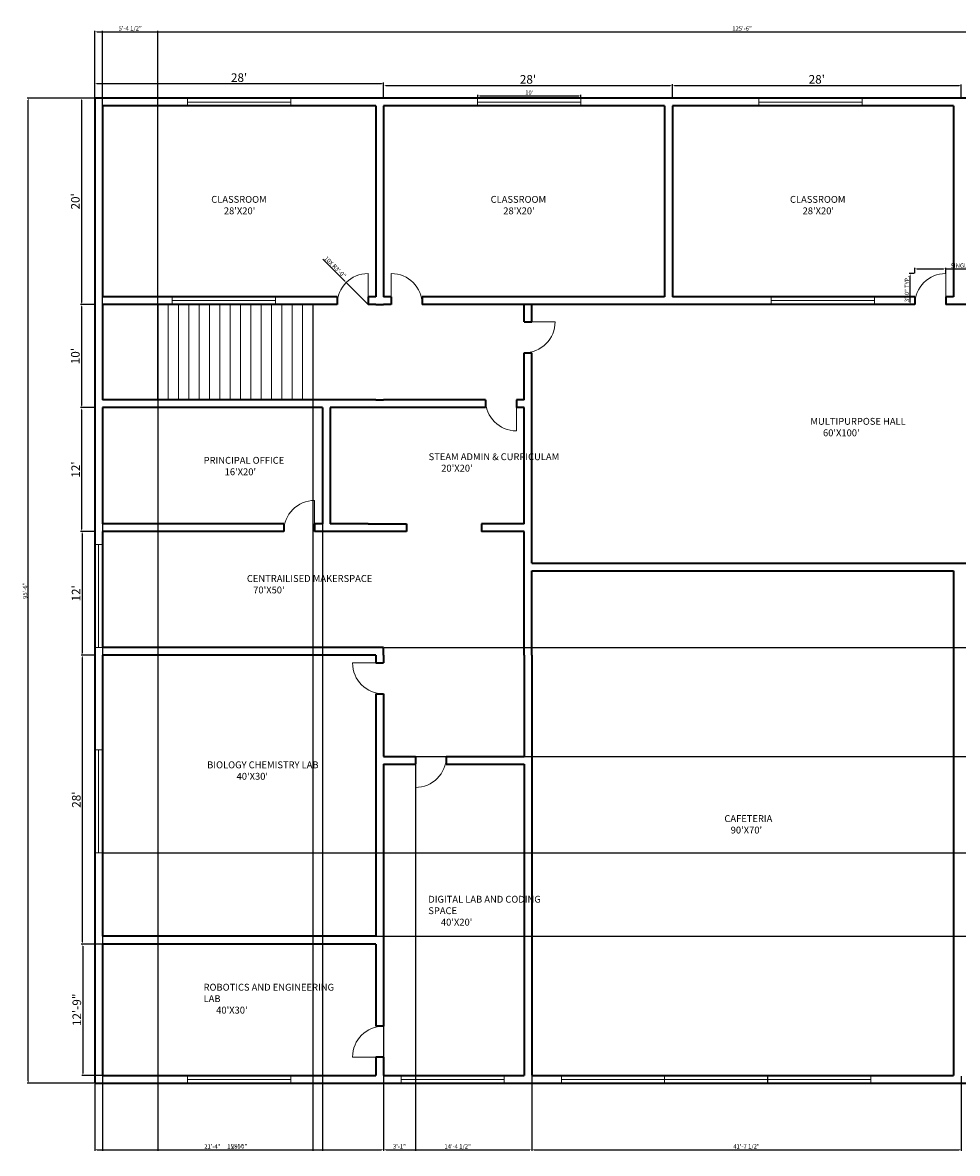
# Model space of a CAD drawing. Units: inches. Extents: x 2394 to 4066, y 1878 to 3193.
# Tile 1 of 3: x 2394 to 3482, y 1878 to 3193. Entities that reach past the tile are written whole.
import ezdxf

# ---------------------------------------------------------------- set-up
doc = ezdxf.new("R2010")
doc.units = ezdxf.units.IN
for name, color, linetype, lineweight in [('A-ANNO-DIMS', 2, 'Continuous', 13), ('A-AREA-IDEN', 7, 'Continuous', 18), ('A-DOOR', 3, 'Continuous', 18), ('A-FLOR-STRS', 8, 'Continuous', 18), ('A-GLAZ', 4, 'Continuous', 18), ('A-WALL', 7, 'Continuous', 35)]:
    doc.layers.add(name, color=color, linetype=linetype, lineweight=lineweight)
doc.styles.get("Standard").update_dxf_attribs({"font": 'arial.ttf'})
doc.dimstyles.new('ISO-25', dxfattribs={"dimtxt": 5, "dimasz": 2.5, "dimexe": 1.25, "dimexo": 0.625, "dimtad": 1, "dimlunit": 3, "dimtxsty": 'Standard', "dimcen": 2.5, "dimadec": 0, "dimazin": 0, "dimtfac": 1, "dimtmove": 0, "dimatfit": 3, "dimfxl": 1, "dimarcsym": 0})

# ---------------------------------------------------------------- blocks, each defined once
blk = doc.blocks.new('*D1')
at = {"layer": 'A-ANNO-DIMS', "color": 0, "lineweight": -2, "transparency": 16777216}
for p, q in [((2478.1, 3105.7), (2478.1, 3123.2)), ((2480.6, 3122), (2811.6, 3122)), ((2814.1, 3105.7), (2814.1, 3123.2))]:
    blk.add_line(p, q, dxfattribs=at)
at = {"layer": 'A-ANNO-DIMS', "color": 0, "transparency": 16777216}
for points in [[(2480.6, 3122.4), (2480.6, 3121.6), (2478.1, 3122)], [(2811.6, 3122.4), (2811.6, 3121.6), (2814.1, 3122)]]:
    blk.add_solid(points, dxfattribs=at)
at = {"layer": 'Defpoints', "color": 0, "transparency": 16777216}
for p in [(2814.1, 3122), (2478.1, 3105.1), (2814.1, 3105.1)]:
    blk.add_point(p, dxfattribs=at)
at = {"layer": 'A-ANNO-DIMS', "color": 0, "transparency": 16777216, "insert": (2646.1, 3127.7), "char_height": 10, "attachment_point": 5}
blk.add_mtext("28'", dxfattribs=at)
blk = doc.blocks.new('*D2')
at = {"layer": 'A-ANNO-DIMS', "color": 0, "lineweight": -2, "transparency": 16777216}
for p, q in [((2814.1, 3105.7), (2814.1, 3121.3)), ((2816.6, 3120), (3147.6, 3120)), ((3150.1, 3105.7), (3150.1, 3121.3))]:
    blk.add_line(p, q, dxfattribs=at)
at = {"layer": 'A-ANNO-DIMS', "color": 0, "transparency": 16777216}
for points in [[(2816.6, 3120.4), (2816.6, 3119.6), (2814.1, 3120)], [(3147.6, 3120.4), (3147.6, 3119.6), (3150.1, 3120)]]:
    blk.add_solid(points, dxfattribs=at)
at = {"layer": 'Defpoints', "color": 0, "transparency": 16777216}
for p in [(3150.1, 3120), (2814.1, 3105.1), (3150.1, 3105.1)]:
    blk.add_point(p, dxfattribs=at)
at = {"layer": 'A-ANNO-DIMS', "color": 0, "transparency": 16777216, "insert": (2982.1, 3125.7), "char_height": 10, "attachment_point": 5}
blk.add_mtext("28'", dxfattribs=at)
blk = doc.blocks.new('*D3')
at = {"layer": 'A-ANNO-DIMS', "color": 0, "lineweight": -2, "transparency": 16777216}
for p, q in [((3150.1, 3105.7), (3150.1, 3121.2)), ((3152.6, 3120), (3483.6, 3120)), ((3486.1, 3105.7), (3486.1, 3121.2))]:
    blk.add_line(p, q, dxfattribs=at)
at = {"layer": 'A-ANNO-DIMS', "color": 0, "transparency": 16777216}
for points in [[(3152.6, 3120.4), (3152.6, 3119.6), (3150.1, 3120)], [(3483.6, 3120.4), (3483.6, 3119.6), (3486.1, 3120)]]:
    blk.add_solid(points, dxfattribs=at)
at = {"layer": 'Defpoints', "color": 0, "transparency": 16777216}
for p in [(3486.1, 3120), (3150.1, 3105.1), (3486.1, 3105.1)]:
    blk.add_point(p, dxfattribs=at)
at = {"layer": 'A-ANNO-DIMS', "color": 0, "transparency": 16777216, "insert": (3318.1, 3125.7), "char_height": 10, "attachment_point": 5}
blk.add_mtext("28'", dxfattribs=at)
blk = doc.blocks.new('*D6')
at = {"layer": 'A-ANNO-DIMS', "color": 0, "lineweight": -2, "transparency": 16777216}
for p, q in [((2477.5, 3105.1), (2461.4, 3105.1)), ((2462.6, 3102.6), (2462.6, 2867.6)), ((2477.5, 2865.1), (2461.4, 2865.1))]:
    blk.add_line(p, q, dxfattribs=at)
at = {"layer": 'A-ANNO-DIMS', "color": 0, "transparency": 16777216}
for points in [[(2462.2, 3102.6), (2463, 3102.6), (2462.6, 3105.1)], [(2462.2, 2867.6), (2463, 2867.6), (2462.6, 2865.1)]]:
    blk.add_solid(points, dxfattribs=at)
at = {"layer": 'Defpoints', "color": 0, "transparency": 16777216}
for p in [(2478.1, 3105.1), (2462.6, 2865.1), (2478.1, 2865.1)]:
    blk.add_point(p, dxfattribs=at)
at = {"layer": 'A-ANNO-DIMS', "color": 0, "transparency": 16777216, "insert": (2456.9, 2985.1), "char_height": 10, "attachment_point": 5, "rotation": 90}
blk.add_mtext("20'", dxfattribs=at)
blk = doc.blocks.new('*D7')
at = {"layer": 'A-ANNO-DIMS', "color": 0, "lineweight": -2, "transparency": 16777216}
for p, q in [((2477.5, 2865.1), (2461.4, 2865.1)), ((2462.6, 2862.6), (2462.6, 2747.6)), ((2477.5, 2745.1), (2461.4, 2745.1))]:
    blk.add_line(p, q, dxfattribs=at)
at = {"layer": 'A-ANNO-DIMS', "color": 0, "transparency": 16777216}
for points in [[(2462.2, 2862.6), (2463, 2862.6), (2462.6, 2865.1)], [(2462.2, 2747.6), (2463, 2747.6), (2462.6, 2745.1)]]:
    blk.add_solid(points, dxfattribs=at)
at = {"layer": 'Defpoints', "color": 0, "transparency": 16777216}
for p in [(2478.1, 2865.1), (2462.6, 2745.1), (2478.1, 2745.1)]:
    blk.add_point(p, dxfattribs=at)
at = {"layer": 'A-ANNO-DIMS', "color": 0, "transparency": 16777216, "insert": (2456.9, 2805.1), "char_height": 10, "attachment_point": 5, "rotation": 90}
blk.add_mtext("10'", dxfattribs=at)
blk = doc.blocks.new('*D8')
at = {"layer": 'A-ANNO-DIMS', "color": 0, "lineweight": -2, "transparency": 16777216}
for p, q in [((2477.5, 2745.1), (2461.7, 2745.1)), ((2462.9, 2742.6), (2462.9, 2603.6)), ((2477.5, 2601.1), (2461.7, 2601.1))]:
    blk.add_line(p, q, dxfattribs=at)
at = {"layer": 'A-ANNO-DIMS', "color": 0, "transparency": 16777216}
for points in [[(2462.5, 2742.6), (2463.3, 2742.6), (2462.9, 2745.1)], [(2462.5, 2603.6), (2463.3, 2603.6), (2462.9, 2601.1)]]:
    blk.add_solid(points, dxfattribs=at)
at = {"layer": 'Defpoints', "color": 0, "transparency": 16777216}
for p in [(2478.1, 2745.1), (2462.9, 2601.1), (2478.1, 2601.1)]:
    blk.add_point(p, dxfattribs=at)
at = {"layer": 'A-ANNO-DIMS', "color": 0, "transparency": 16777216, "insert": (2457.3, 2673.1), "char_height": 10, "attachment_point": 5, "rotation": 90}
blk.add_mtext("12'", dxfattribs=at)
blk = doc.blocks.new('*D9')
at = {"layer": 'A-ANNO-DIMS', "color": 0, "lineweight": -2, "transparency": 16777216}
for p, q in [((2477.5, 2601.1), (2462.2, 2601.1)), ((2463.4, 2598.6), (2463.4, 2459.6)), ((2477.5, 2457.1), (2462.2, 2457.1))]:
    blk.add_line(p, q, dxfattribs=at)
at = {"layer": 'A-ANNO-DIMS', "color": 0, "transparency": 16777216}
for points in [[(2463, 2598.6), (2463.9, 2598.6), (2463.4, 2601.1)], [(2463, 2459.6), (2463.9, 2459.6), (2463.4, 2457.1)]]:
    blk.add_solid(points, dxfattribs=at)
at = {"layer": 'Defpoints', "color": 0, "transparency": 16777216}
for p in [(2478.1, 2601.1), (2463.4, 2457.1), (2478.1, 2457.1)]:
    blk.add_point(p, dxfattribs=at)
at = {"layer": 'A-ANNO-DIMS', "color": 0, "transparency": 16777216, "insert": (2457.8, 2529.1), "char_height": 10, "attachment_point": 5, "rotation": 90}
blk.add_mtext("12'", dxfattribs=at)
blk = doc.blocks.new('*D10')
at = {"layer": 'A-ANNO-DIMS', "color": 0, "lineweight": -2, "transparency": 16777216}
for p, q in [((2477.5, 2457.1), (2462.4, 2457.1)), ((2463.7, 2454.6), (2463.7, 2123.6)), ((2477.5, 2121.1), (2462.4, 2121.1))]:
    blk.add_line(p, q, dxfattribs=at)
at = {"layer": 'A-ANNO-DIMS', "color": 0, "transparency": 16777216}
for points in [[(2463.3, 2454.6), (2464.1, 2454.6), (2463.7, 2457.1)], [(2463.3, 2123.6), (2464.1, 2123.6), (2463.7, 2121.1)]]:
    blk.add_solid(points, dxfattribs=at)
at = {"layer": 'Defpoints', "color": 0, "transparency": 16777216}
for p in [(2478.1, 2457.1), (2463.7, 2121.1), (2478.1, 2121.1)]:
    blk.add_point(p, dxfattribs=at)
at = {"layer": 'A-ANNO-DIMS', "color": 0, "transparency": 16777216, "insert": (2458, 2289.1), "char_height": 10, "attachment_point": 5, "rotation": 90}
blk.add_mtext("28'", dxfattribs=at)
blk = doc.blocks.new('*D11')
at = {"layer": 'A-ANNO-DIMS', "color": 0, "lineweight": -2, "transparency": 16777216}
for p, q in [((2486.5, 2121.1), (2463, 2121.1)), ((2464.3, 2118.6), (2464.3, 1970.6)), ((2486.5, 1968.1), (2463, 1968.1))]:
    blk.add_line(p, q, dxfattribs=at)
at = {"layer": 'A-ANNO-DIMS', "color": 0, "transparency": 16777216}
for points in [[(2463.9, 2118.6), (2464.7, 2118.6), (2464.3, 2121.1)], [(2463.9, 1970.6), (2464.7, 1970.6), (2464.3, 1968.1)]]:
    blk.add_solid(points, dxfattribs=at)
at = {"layer": 'Defpoints', "color": 0, "transparency": 16777216}
for p in [(2487.1, 2121.1), (2464.3, 1968.1), (2487.1, 1968.1)]:
    blk.add_point(p, dxfattribs=at)
at = {"layer": 'A-ANNO-DIMS', "color": 0, "transparency": 16777216, "insert": (2458.6, 2044.6), "char_height": 10, "attachment_point": 5, "rotation": 90}
blk.add_mtext('12\'-9"', dxfattribs=at)
blk = doc.blocks.new('*D12')
at = {"layer": 'A-ANNO-DIMS', "color": 0, "lineweight": -2, "transparency": 16777216}
for p, q in [((2923.6, 3105.7), (2923.6, 3109)), ((2926.1, 3107.8), (3041.1, 3107.8)), ((3043.6, 3105.7), (3043.6, 3109))]:
    blk.add_line(p, q, dxfattribs=at)
at = {"layer": 'A-ANNO-DIMS', "color": 0, "transparency": 16777216}
for points in [[(2926.1, 3108.2), (2926.1, 3107.3), (2923.6, 3107.8)], [(3041.1, 3108.2), (3041.1, 3107.3), (3043.6, 3107.8)]]:
    blk.add_solid(points, dxfattribs=at)
at = {"layer": 'Defpoints', "color": 0, "transparency": 16777216}
for p in [(2923.6, 3105.1), (3043.6, 3107.8), (3043.6, 3105.1)]:
    blk.add_point(p, dxfattribs=at)
at = {"layer": 'A-ANNO-DIMS', "color": 0, "transparency": 16777216, "insert": (2983.6, 3110.9), "char_height": 5, "attachment_point": 5}
blk.add_mtext("10'", dxfattribs=at)
blk = doc.blocks.new('DOOR-SINGLE-36IN')
blk.add_line((36, 0), (36, 36))
blk.add_arc((36, 0), 36, 90, 180)
blk = doc.blocks.new('WINDOW-120IN')
for p, q in [((0, 0), (0, 9)), ((120, 4.5), (0, 4.5)), ((120, 0), (120, 9))]:
    blk.add_line(p, q)
blk = doc.blocks.new('*D15')
at = {"layer": 'A-ANNO-DIMS', "color": 0, "lineweight": -2, "transparency": 16777216}
for p, q in [((3432.1, 2901.7), (3432.1, 2907.7)), ((3468.1, 2901.7), (3468.1, 2907.7)), ((3434.6, 2906.5), (3465.6, 2906.5)), ((3468.1, 2906.5), (3552.8, 2906.5))]:
    blk.add_line(p, q, dxfattribs=at)
at = {"layer": 'A-ANNO-DIMS', "color": 0, "transparency": 16777216}
for points in [[(3434.6, 2906.9), (3434.6, 2906.1), (3432.1, 2906.5)], [(3465.6, 2906.9), (3465.6, 2906.1), (3468.1, 2906.5)]]:
    blk.add_solid(points, dxfattribs=at)
at = {"layer": 'Defpoints', "color": 0, "transparency": 16777216}
for p in [(3432.1, 2901.1), (3468.1, 2906.5), (3468.1, 2901.1)]:
    blk.add_point(p, dxfattribs=at)
at = {"layer": 'A-ANNO-DIMS', "color": 0, "transparency": 16777216, "insert": (3511.7, 2909.7), "char_height": 5, "attachment_point": 5}
blk.add_mtext('SINGLE DOOR 3\'-0" TYP.', dxfattribs=at)
blk = doc.blocks.new('*D16')
at = {"layer": 'A-ANNO-DIMS', "color": 0, "lineweight": -2, "transparency": 16777216}
for p, q in [((3431.5, 2901.1), (3425.4, 2901.1)), ((3426.7, 2867.6), (3426.7, 2898.6)), ((3431.5, 2865.1), (3425.4, 2865.1))]:
    blk.add_line(p, q, dxfattribs=at)
at = {"layer": 'A-ANNO-DIMS', "color": 0, "transparency": 16777216}
for points in [[(3426.3, 2898.6), (3427.1, 2898.6), (3426.7, 2901.1)], [(3426.3, 2867.6), (3427.1, 2867.6), (3426.7, 2865.1)]]:
    blk.add_solid(points, dxfattribs=at)
at = {"layer": 'Defpoints', "color": 0, "transparency": 16777216}
for p in [(3426.7, 2901.1), (3432.1, 2901.1), (3432.1, 2865.1)]:
    blk.add_point(p, dxfattribs=at)
at = {"layer": 'A-ANNO-DIMS', "color": 0, "transparency": 16777216, "insert": (3423.5, 2883.1), "char_height": 5, "attachment_point": 5, "rotation": 90}
blk.add_mtext('3\'-0" TYP.', dxfattribs=at)
blk = doc.blocks.new('*D19')
at = {"layer": 'A-ANNO-DIMS', "color": 0, "lineweight": -2, "transparency": 16777216}
for p, q in [((2478.1, 3105.7), (2478.1, 3183.6)), ((3984.1, 3105.7), (3984.1, 3183.6)), ((2480.6, 3182.3), (3981.6, 3182.3))]:
    blk.add_line(p, q, dxfattribs=at)
at = {"layer": 'A-ANNO-DIMS', "color": 0, "transparency": 16777216}
for points in [[(2480.6, 3182.8), (2480.6, 3181.9), (2478.1, 3182.3)], [(3981.6, 3182.8), (3981.6, 3181.9), (3984.1, 3182.3)]]:
    blk.add_solid(points, dxfattribs=at)
at = {"layer": 'Defpoints', "color": 0, "transparency": 16777216}
for p in [(3984.1, 3182.3), (2478.1, 3105.1), (3984.1, 3105.1)]:
    blk.add_point(p, dxfattribs=at)
at = {"layer": 'A-ANNO-DIMS', "color": 0, "transparency": 16777216, "insert": (3231.1, 3185.5), "char_height": 5, "attachment_point": 5}
blk.add_mtext('125\'-6"', dxfattribs=at)
blk = doc.blocks.new('*D20')
at = {"layer": 'A-ANNO-DIMS', "color": 0, "lineweight": -2, "transparency": 16777216}
for p, q in [((2477.5, 3105.1), (2399.6, 3105.1)), ((2400.8, 1961.6), (2400.8, 3102.6)), ((2477.5, 1959.1), (2399.6, 1959.1))]:
    blk.add_line(p, q, dxfattribs=at)
at = {"layer": 'A-ANNO-DIMS', "color": 0, "transparency": 16777216}
for points in [[(2400.4, 3102.6), (2401.3, 3102.6), (2400.8, 3105.1)], [(2400.4, 1961.6), (2401.3, 1961.6), (2400.8, 1959.1)]]:
    blk.add_solid(points, dxfattribs=at)
at = {"layer": 'Defpoints', "color": 0, "transparency": 16777216}
for p in [(2400.8, 3105.1), (2478.1, 3105.1), (2478.1, 1959.1)]:
    blk.add_point(p, dxfattribs=at)
at = {"layer": 'A-ANNO-DIMS', "color": 0, "transparency": 16777216, "insert": (2397.7, 2532.1), "char_height": 5, "attachment_point": 5, "rotation": 90}
blk.add_mtext('95\'-6"', dxfattribs=at)
blk = doc.blocks.new('*D21')
at = {"layer": 'A-ANNO-DIMS', "color": 0, "lineweight": -2, "transparency": 16777216}
for p, q in [((2814.1, 1967.5), (2814.1, 1880.6)), ((2478.1, 1958.5), (2478.1, 1880.6)), ((2480.6, 1881.8), (2811.6, 1881.8))]:
    blk.add_line(p, q, dxfattribs=at)
at = {"layer": 'A-ANNO-DIMS', "color": 0, "transparency": 16777216}
for points in [[(2480.6, 1882.3), (2480.6, 1881.4), (2478.1, 1881.8)], [(2811.6, 1882.3), (2811.6, 1881.4), (2814.1, 1881.8)]]:
    blk.add_solid(points, dxfattribs=at)
at = {"layer": 'Defpoints', "color": 0, "transparency": 16777216}
for p in [(2814.1, 1968.1), (2478.1, 1959.1), (2814.1, 1881.8)]:
    blk.add_point(p, dxfattribs=at)
at = {"layer": 'A-ANNO-DIMS', "color": 0, "transparency": 16777216, "insert": (2646.1, 1885), "char_height": 5, "attachment_point": 5}
blk.add_mtext('28\'-0"', dxfattribs=at)
blk = doc.blocks.new('*D22')
at = {"layer": 'A-ANNO-DIMS', "color": 0, "lineweight": -2, "transparency": 16777216}
for p, q in [((2814.1, 1967.5), (2814.1, 1880.6)), ((2986.6, 1967.5), (2986.6, 1880.6)), ((2816.6, 1881.8), (2984.1, 1881.8))]:
    blk.add_line(p, q, dxfattribs=at)
at = {"layer": 'A-ANNO-DIMS', "color": 0, "transparency": 16777216}
for points in [[(2816.6, 1882.3), (2816.6, 1881.4), (2814.1, 1881.8)], [(2984.1, 1882.3), (2984.1, 1881.4), (2986.6, 1881.8)]]:
    blk.add_solid(points, dxfattribs=at)
at = {"layer": 'Defpoints', "color": 0, "transparency": 16777216}
for p in [(2814.1, 1968.1), (2986.6, 1968.1), (2986.6, 1881.8)]:
    blk.add_point(p, dxfattribs=at)
at = {"layer": 'A-ANNO-DIMS', "color": 0, "transparency": 16777216, "insert": (2900.3, 1885.1), "char_height": 5, "attachment_point": 5}
blk.add_mtext('14\'-4 1/2"', dxfattribs=at)
blk = doc.blocks.new('*D23')
at = {"layer": 'A-ANNO-DIMS', "color": 0, "lineweight": -2, "transparency": 16777216}
for p, q in [((2986.6, 1967.5), (2986.6, 1880.6)), ((3486.1, 1967.5), (3486.1, 1880.6)), ((2989.1, 1881.8), (3483.6, 1881.8))]:
    blk.add_line(p, q, dxfattribs=at)
at = {"layer": 'A-ANNO-DIMS', "color": 0, "transparency": 16777216}
for points in [[(2989.1, 1882.3), (2989.1, 1881.4), (2986.6, 1881.8)], [(3483.6, 1882.3), (3483.6, 1881.4), (3486.1, 1881.8)]]:
    blk.add_solid(points, dxfattribs=at)
at = {"layer": 'Defpoints', "color": 0, "transparency": 16777216}
for p in [(2986.6, 1968.1), (3486.1, 1968.1), (3486.1, 1881.8)]:
    blk.add_point(p, dxfattribs=at)
at = {"layer": 'A-ANNO-DIMS', "color": 0, "transparency": 16777216, "insert": (3236.3, 1885.1), "char_height": 5, "attachment_point": 5}
blk.add_mtext('41\'-7 1/2"', dxfattribs=at)
blk = doc.blocks.new('*D29')
at = {"layer": 'A-ANNO-DIMS', "color": 0, "lineweight": -2, "transparency": 16777216}
for p, q in [((2814.7, 2466.1), (4062.6, 2466.1)), ((4061.3, 2463.6), (4061.3, 2341.8)), ((2814.7, 2339.3), (4062.6, 2339.3))]:
    blk.add_line(p, q, dxfattribs=at)
at = {"layer": 'A-ANNO-DIMS', "color": 0, "transparency": 16777216}
for points in [[(4060.9, 2463.6), (4061.8, 2463.6), (4061.3, 2466.1)], [(4060.9, 2341.8), (4061.8, 2341.8), (4061.3, 2339.3)]]:
    blk.add_solid(points, dxfattribs=at)
at = {"layer": 'Defpoints', "color": 0, "transparency": 16777216}
for p in [(2814.1, 2466.1), (2814.1, 2339.3), (4061.3, 2339.3)]:
    blk.add_point(p, dxfattribs=at)
at = {"layer": 'A-ANNO-DIMS', "color": 0, "transparency": 16777216, "insert": (4058.2, 2402.7), "char_height": 5, "attachment_point": 5, "rotation": 90}
blk.add_mtext('10\'-7"', dxfattribs=at)
blk = doc.blocks.new('*D30')
at = {"layer": 'A-ANNO-DIMS', "color": 0, "lineweight": -2, "transparency": 16777216}
for p, q in [((2487.1, 2744.5), (2487.1, 1880.6)), ((2743, 2744.5), (2743, 1880.6)), ((2489.6, 1881.8), (2740.5, 1881.8))]:
    blk.add_line(p, q, dxfattribs=at)
at = {"layer": 'A-ANNO-DIMS', "color": 0, "transparency": 16777216}
for points in [[(2489.6, 1882.3), (2489.6, 1881.4), (2487.1, 1881.8)], [(2740.5, 1882.3), (2740.5, 1881.4), (2743, 1881.8)]]:
    blk.add_solid(points, dxfattribs=at)
at = {"layer": 'Defpoints', "color": 0, "transparency": 16777216}
for p in [(2487.1, 2745.1), (2743, 2745.1), (2743, 1881.8)]:
    blk.add_point(p, dxfattribs=at)
at = {"layer": 'A-ANNO-DIMS', "color": 0, "transparency": 16777216, "insert": (2615, 1885), "char_height": 5, "attachment_point": 5}
blk.add_mtext('21\'-4"', dxfattribs=at)
blk = doc.blocks.new('*D31')
at = {"layer": 'A-ANNO-DIMS', "color": 0, "lineweight": -2, "transparency": 16777216}
for p, q in [((2487.1, 2754.7), (2487.1, 3183.6)), ((2551.7, 2754.7), (2551.7, 3183.6)), ((2489.6, 3182.3), (2549.2, 3182.3))]:
    blk.add_line(p, q, dxfattribs=at)
at = {"layer": 'A-ANNO-DIMS', "color": 0, "transparency": 16777216}
for points in [[(2489.6, 3182.8), (2489.6, 3181.9), (2487.1, 3182.3)], [(2549.2, 3182.8), (2549.2, 3181.9), (2551.7, 3182.3)]]:
    blk.add_solid(points, dxfattribs=at)
at = {"layer": 'Defpoints', "color": 0, "transparency": 16777216}
for p in [(2551.7, 3182.3), (2487.1, 2754.1), (2551.7, 2754.1)]:
    blk.add_point(p, dxfattribs=at)
at = {"layer": 'A-ANNO-DIMS', "color": 0, "transparency": 16777216, "insert": (2519.4, 3185.6), "char_height": 5, "attachment_point": 5}
blk.add_mtext('5\'-4 1/2"', dxfattribs=at)
blk = doc.blocks.new('*D32')
at = {"layer": 'A-ANNO-DIMS', "color": 0, "lineweight": -2, "transparency": 16777216}
for p, q in [((2551.7, 2864.5), (2551.7, 1880.6)), ((2731.7, 2864.5), (2731.7, 1880.6)), ((2554.2, 1881.8), (2729.2, 1881.8))]:
    blk.add_line(p, q, dxfattribs=at)
at = {"layer": 'A-ANNO-DIMS', "color": 0, "transparency": 16777216}
for points in [[(2554.2, 1882.3), (2554.2, 1881.4), (2551.7, 1881.8)], [(2729.2, 1882.3), (2729.2, 1881.4), (2731.7, 1881.8)]]:
    blk.add_solid(points, dxfattribs=at)
at = {"layer": 'Defpoints', "color": 0, "transparency": 16777216}
for p in [(2551.7, 2865.1), (2731.7, 2865.1), (2731.7, 1881.8)]:
    blk.add_point(p, dxfattribs=at)
at = {"layer": 'A-ANNO-DIMS', "color": 0, "transparency": 16777216, "insert": (2641.7, 1885), "char_height": 5, "attachment_point": 5}
blk.add_mtext('15\'-0"', dxfattribs=at)
blk = doc.blocks.new('*D34')
at = {"layer": 'A-ANNO-DIMS', "color": 0, "lineweight": -2, "transparency": 16777216}
for p, q in [((2487.7, 2227.2), (4062.6, 2227.2)), ((4061.3, 2132.6), (4061.3, 2224.7)), ((2487.7, 2130.1), (4062.6, 2130.1))]:
    blk.add_line(p, q, dxfattribs=at)
at = {"layer": 'A-ANNO-DIMS', "color": 0, "transparency": 16777216}
for points in [[(4060.9, 2224.7), (4061.8, 2224.7), (4061.3, 2227.2)], [(4060.9, 2132.6), (4061.8, 2132.6), (4061.3, 2130.1)]]:
    blk.add_solid(points, dxfattribs=at)
at = {"layer": 'Defpoints', "color": 0, "transparency": 16777216}
for p in [(2487.1, 2227.2), (4061.3, 2227.2), (2487.1, 2130.1)]:
    blk.add_point(p, dxfattribs=at)
at = {"layer": 'A-ANNO-DIMS', "color": 0, "transparency": 16777216, "insert": (4058.2, 2178.7), "char_height": 5, "attachment_point": 5, "rotation": 90}
blk.add_mtext('8\'-1"', dxfattribs=at)
blk = doc.blocks.new('*D35')
at = {"layer": 'A-ANNO-DIMS', "color": 0, "lineweight": -2, "transparency": 16777216}
for p, q in [((2814.1, 2329.6), (2814.1, 1880.6)), ((2851.1, 2329.6), (2851.1, 1880.6)), ((2816.6, 1881.8), (2848.6, 1881.8))]:
    blk.add_line(p, q, dxfattribs=at)
at = {"layer": 'A-ANNO-DIMS', "color": 0, "transparency": 16777216}
for points in [[(2816.6, 1882.3), (2816.6, 1881.4), (2814.1, 1881.8)], [(2848.6, 1882.3), (2848.6, 1881.4), (2851.1, 1881.8)]]:
    blk.add_solid(points, dxfattribs=at)
at = {"layer": 'Defpoints', "color": 0, "transparency": 16777216}
for p in [(2814.1, 2330.3), (2851.1, 2330.3), (2851.1, 1881.8)]:
    blk.add_point(p, dxfattribs=at)
at = {"layer": 'A-ANNO-DIMS', "color": 0, "transparency": 16777216, "insert": (2832.6, 1885), "char_height": 5, "attachment_point": 5}
blk.add_mtext('3\'-1"', dxfattribs=at)
blk = doc.blocks.new('*D37')
at = {"layer": 'A-ANNO-DIMS', "color": 0, "lineweight": -2, "transparency": 16777216}
for p, q in [((2743.4, 2917.8), (2768.9, 2892.3)), ((2796.1, 2865.1), (2770.6, 2890.5))]:
    blk.add_line(p, q, dxfattribs=at)
at = {"layer": 'A-ANNO-DIMS', "color": 0, "transparency": 16777216}
blk.add_solid([(2769.2, 2892.6), (2768.6, 2892), (2770.6, 2890.5)], dxfattribs=at)
at = {"layer": 'Defpoints', "color": 0, "transparency": 16777216}
for p in [(2770.6, 2890.5), (2796.1, 2865.1)]:
    blk.add_point(p, dxfattribs=at)
at = {"layer": 'A-ANNO-DIMS', "color": 0, "transparency": 16777216, "insert": (2757.5, 2908.2), "char_height": 5, "attachment_point": 5, "rotation": 314.9996}
blk.add_mtext('10X R3\'-0"', dxfattribs=at)

msp = doc.modelspace()

# ---------------------------------------------------------------- linework, layer by layer
at = {"layer": 'A-FLOR-STRS'}
for p, q in [((2551.717, 2865.092), (2551.717, 2754.092)), ((2563.717, 2865.092), (2563.717, 2754.092)), ((2575.717, 2865.092), (2575.717, 2754.092)), ((2587.717, 2865.092), (2587.717, 2754.092)), ((2599.717, 2865.092), (2599.717, 2754.092)), ((2611.717, 2865.092), (2611.717, 2754.092)), ((2623.717, 2865.092), (2623.717, 2754.092)), ((2635.717, 2865.092), (2635.717, 2754.092)), ((2647.717, 2865.092), (2647.717, 2754.092)), ((2659.717, 2865.092), (2659.717, 2754.092)), ((2671.717, 2865.092), (2671.717, 2754.092)), ((2683.717, 2865.092), (2683.717, 2754.092)), ((2695.717, 2865.092), (2695.717, 2754.092)), ((2707.717, 2865.092), (2707.717, 2754.092)), ((2719.717, 2865.092), (2719.717, 2754.092)), ((2731.717, 2865.092), (2731.717, 2754.092))]:
    msp.add_line(p, q, dxfattribs=at)
at = {"layer": 'A-GLAZ'}
msp.add_line((3141.098, 1968.092), (3141.098, 1959.092), dxfattribs=at)
at = {"layer": 'A-WALL'}
for p, q in [((3984.098, 3105.092), (2478.098, 3105.092)), ((2478.098, 3105.092), (2478.098, 1959.092)), ((2487.098, 3096.092), (2487.098, 2874.092)), ((2805.098, 3096.092), (2487.098, 3096.092)), ((2805.098, 3096.092), (2805.098, 2874.092)), ((2814.098, 3096.092), (2814.098, 2874.092)), ((3141.098, 3096.092), (2814.098, 3096.092)), ((3141.098, 3096.092), (3141.098, 2874.092)), ((3150.098, 3096.092), (3150.098, 2874.092)), ((3477.098, 3096.092), (3150.098, 3096.092)), ((3477.098, 3096.092), (3477.098, 2874.092)), ((2760.098, 2874.092), (2487.098, 2874.092)), ((2760.098, 2874.092), (2760.098, 2865.092)), ((2796.098, 2874.092), (2796.098, 2865.092)), ((2805.098, 2874.092), (2796.098, 2874.092)), ((2823.098, 2874.092), (2814.098, 2874.092)), ((2823.098, 2874.092), (2823.098, 2865.092)), ((3141.098, 2874.092), (2859.098, 2874.092)), ((2859.098, 2874.092), (2859.098, 2865.092)), ((3432.098, 2874.092), (3150.098, 2874.092)), ((3432.098, 2874.092), (3432.098, 2865.092)), ((3477.098, 2874.092), (3468.098, 2874.092)), ((3468.098, 2874.092), (3468.098, 2865.092)), ((2760.098, 2865.092), (2487.098, 2865.092)), ((2487.098, 2865.092), (2487.098, 2754.092)), ((2805.098, 2865.092), (2796.098, 2865.092)), ((2805.098, 2865.092), (2814.098, 2865.092)), ((2823.098, 2865.092), (2814.098, 2865.092)), ((3432.098, 2865.092), (2859.098, 2865.092)), ((2977.598, 2844.901), (2977.598, 2865.092)), ((2986.598, 2844.901), (2986.598, 2865.092)), ((3576.098, 2865.092), (3468.098, 2865.092)), ((2977.598, 2844.901), (2986.598, 2844.901)), ((2977.598, 2754.092), (2977.598, 2808.901)), ((2977.598, 2808.901), (2986.598, 2808.901)), ((2986.598, 2564.327), (2986.598, 2808.901)), ((2805.098, 2754.092), (2487.098, 2754.092)), ((2805.098, 2754.092), (2814.098, 2754.092)), ((2932.598, 2754.092), (2814.098, 2754.092)), ((2932.598, 2754.092), (2932.598, 2745.092)), ((2977.598, 2754.092), (2968.598, 2754.092)), ((2968.598, 2754.092), (2968.598, 2745.092)), ((2487.098, 2745.092), (2487.098, 2610.092)), ((2742.957, 2745.092), (2487.098, 2745.092)), ((2742.957, 2745.092), (2742.957, 2610.092)), ((2932.598, 2745.092), (2751.957, 2745.092)), ((2751.957, 2745.092), (2751.957, 2610.092)), ((2932.598, 2745.092), (2814.098, 2745.092)), ((2977.598, 2745.092), (2968.598, 2745.092)), ((2977.598, 2610.092), (2977.598, 2745.092)), ((2697.957, 2610.092), (2487.098, 2610.092)), ((2697.957, 2610.092), (2697.957, 2601.092)), ((2742.957, 2610.092), (2733.957, 2610.092)), ((2733.957, 2610.092), (2733.957, 2601.092)), ((2760.098, 2610.092), (2751.957, 2610.092)), ((2796.098, 2610.092), (2760.098, 2610.092)), ((2796.098, 2610.092), (2840.829, 2610.092)), ((2840.829, 2610.092), (2840.829, 2601.092)), ((2977.598, 2610.092), (2928.098, 2610.092)), ((2928.098, 2610.092), (2928.098, 2601.092)), ((2487.098, 2601.092), (2487.098, 2466.092)), ((2697.957, 2601.092), (2487.098, 2601.092)), ((2760.098, 2601.092), (2733.957, 2601.092)), ((2796.098, 2601.092), (2760.098, 2601.092)), ((2840.829, 2601.092), (2796.098, 2601.092)), ((2977.598, 2601.092), (2928.098, 2601.092)), ((2977.598, 2457.092), (2977.598, 2601.092)), ((2986.598, 2564.327), (3698.204, 2564.327)), ((2986.598, 2457.092), (2986.598, 2555.327)), ((2986.598, 2555.327), (3477.098, 2555.327)), ((3477.098, 2555.327), (3477.098, 1968.092)), ((2814.098, 2466.092), (2487.098, 2466.092)), ((2814.098, 2457.092), (2814.098, 2466.092)), ((2805.098, 2457.092), (2487.098, 2457.092)), ((2487.098, 2457.092), (2487.098, 2130.092)), ((2805.098, 2457.092), (2805.098, 2448.092)), ((2805.098, 2448.092), (2814.098, 2448.092)), ((2814.098, 2457.092), (2814.098, 2448.092)), ((2977.598, 2457.092), (2977.598, 2339.252)), ((2986.598, 2457.092), (2986.598, 1968.092)), ((2805.098, 2412.092), (2814.098, 2412.092)), ((2805.098, 2412.092), (2805.098, 2130.092)), ((2814.098, 2412.092), (2814.098, 2339.252)), ((2814.098, 2339.252), (2851.094, 2339.252)), ((2814.098, 2330.252), (2851.094, 2330.252)), ((2814.098, 2330.252), (2814.098, 2130.092)), ((2851.094, 2339.252), (2851.094, 2330.252)), ((2887.094, 2339.252), (2887.094, 2330.252)), ((2887.094, 2339.252), (2977.598, 2339.252)), ((2887.094, 2330.252), (2977.598, 2330.252)), ((2977.598, 2330.252), (2977.598, 2130.092)), ((2805.098, 2130.092), (2487.098, 2130.092)), ((2805.098, 2121.092), (2487.098, 2121.092)), ((2487.098, 2121.092), (2487.098, 1968.092)), ((2805.098, 2121.092), (2805.098, 2025.694)), ((2814.098, 2130.092), (2814.098, 2121.092)), ((2814.098, 2121.092), (2814.098, 2025.694)), ((2977.598, 2130.092), (2977.598, 2121.092)), ((2977.598, 2121.092), (2977.598, 1968.092)), ((2814.098, 2025.694), (2805.098, 2025.694)), ((2814.098, 1989.694), (2805.098, 1989.694)), ((2805.098, 1989.694), (2805.098, 1968.092)), ((2814.098, 1989.694), (2814.098, 1968.092)), ((2487.098, 1968.092), (2805.098, 1968.092)), ((2814.098, 1968.092), (2977.598, 1968.092)), ((2814.098, 1968.092), (2977.598, 1968.092)), ((2986.598, 1968.092), (3477.098, 1968.092)), ((2478.098, 1959.092), (3984.098, 1959.092))]:
    msp.add_line(p, q, dxfattribs=at)

# ---------------------------------------------------------------- block references
at = {"layer": 'A-DOOR'}
for p in [(2760.098, 2865.092), (3432.098, 2865.092), (2697.958, 2601.092)]:
    msp.add_blockref('DOOR-SINGLE-36IN', p, dxfattribs=at)
at = {"layer": 'A-DOOR', "extrusion": (0, 0, -1), "zscale": -1}
msp.add_blockref('DOOR-SINGLE-36IN', (-2859.097, 2865.092), dxfattribs=at)
for p, rotation in [((-2977.598, 2808.902), 89.99999999999999), ((-2932.598, 2754.092), 180), ((-2814.098, 2025.693), 269.9999999999994)]:
    msp.add_blockref('DOOR-SINGLE-36IN', p, dxfattribs=dict(at, rotation=rotation))
at = {"layer": 'A-DOOR'}
for p, rotation in [((2814.098, 2412.092), 89.99999999999928), ((2887.094, 2339.252), 180)]:
    msp.add_blockref('DOOR-SINGLE-36IN', p, dxfattribs=dict(at, rotation=rotation))
at = {"layer": 'A-GLAZ'}
msp.add_blockref('WINDOW-120IN', (2586.098, 3096.092), dxfattribs=at)
for p, rotation in [((3043.58, 3105.092), 180), ((3370.771, 3105.092), 180), ((2688.384, 2874.092), 180), ((3385.144, 2874.092), 180), ((2487.098, 2466.092), 89.9999999999996), ((2487.098, 2227.221), 89.99999999999999), ((2706.097, 1968.092), 180), ((2954.425, 1968.092), 180), ((3141.097, 1968.092), 180), ((3260.809, 1968.092), 180), ((3381.047, 1968.092), 180)]:
    msp.add_blockref('WINDOW-120IN', p, dxfattribs=dict(at, rotation=rotation))

# ---------------------------------------------------------------- texts
at = {"layer": 'A-AREA-IDEN', "char_height": 8, "attachment_point": 1}
for s, insert in [("CLASSROOM\\P      28'X20'", (2613.684, 2991.385)), ("CLASSROOM\\P      28'X20'", (2938.682, 2991.385)), ("CLASSROOM\\P      28'X20'", (3286.879, 2991.385)), ("MULTIPURPOSE HALL\\P      60'X100'", (3310.607, 2733.168)), ("PRINCIPAL OFFICE\\P          16'X20'", (2604.827, 2687.82)), ("STEAM ADMIN & CURRICULAM\\P      20'X20'", (2866.535, 2692.015)), ("CENTRAILISED MAKERSPACE\\P   70'X50'", (2655.126, 2550.333)), ("BIOLOGY CHEMISTRY LAB\\P              40'X30'", (2608.943, 2333.59)), ("CAFETERIA\\P   90'X70'", (3210.568, 2271.055)), ("DIGITAL LAB AND CODING SPACE\\P      40'X20'", (2866.164, 2177.238)), ("ROBOTICS AND ENGINEERING LAB\\P      40'X30'", (2604.744, 2074.897))]:
    msp.add_mtext_dynamic_manual_height_columns(s, width=162.41234, gutter_width=12.5, heights=[0], dxfattribs=dict(at, insert=insert))

# ---------------------------------------------------------------- dimensions: what is measured, and where the dimension line sits
at = {"layer": 'A-ANNO-DIMS'}
for base, p1, p2, override, picture, middle in [((3984.098, 3182.342), (2478.098, 3105.092), (3984.098, 3105.092), {"dimdec": 1, "dimlfac": 1, "dimrnd": 0, "dimzin": 1, "dimdsep": 46, "dimlunit": 4, "dimfrac": 2}, '*D19', (3231.098, 3185.52)), ((2551.717, 3182.342), (2487.098, 2754.092), (2551.717, 2754.092), {"dimdec": 1, "dimlfac": 1, "dimrnd": 0, "dimzin": 1, "dimdsep": 46, "dimlunit": 4, "dimfrac": 2}, '*D31', (2519.407, 3185.552)), ((2814.098, 3121.972), (2478.098, 3105.092), (2814.098, 3105.092), {"dimtxt": 10, "dimclrd": 0, "dimclre": 0, "dimclrt": 0}, '*D1', (2646.098, 3127.702)), ((3150.098, 3120.001), (2814.098, 3105.092), (3150.098, 3105.092), {"dimtxt": 10, "dimclrd": 0, "dimclre": 0, "dimclrt": 0}, '*D2', (2982.098, 3125.731)), ((3486.098, 3119.972), (3150.098, 3105.092), (3486.098, 3105.092), {"dimtxt": 10, "dimclrd": 0, "dimclre": 0, "dimclrt": 0}, '*D3', (3318.098, 3125.703)), ((3043.581, 3107.756), (2923.581, 3105.092), (3043.581, 3105.092), {"dimclrd": 0, "dimclre": 0, "dimclrt": 0}, '*D12', (2983.581, 3110.934)), ((2731.717, 1881.842), (2551.717, 2865.092), (2731.717, 2865.092), {"dimdec": 1, "dimlfac": 1, "dimrnd": 0, "dimzin": 1, "dimdsep": 46, "dimlunit": 4, "dimfrac": 2}, '*D32', (2641.717, 1885.02)), ((2742.957, 1881.842), (2487.098, 2745.092), (2742.957, 2745.092), {"dimdec": 1, "dimlfac": 1, "dimrnd": 0, "dimzin": 1, "dimdsep": 46, "dimlunit": 4, "dimfrac": 2}, '*D30', (2615.027, 1884.977)), ((2851.094, 1881.842), (2814.098, 2330.252), (2851.094, 2330.252), {"dimdec": 1, "dimlfac": 1, "dimrnd": 0, "dimzin": 1, "dimdsep": 46, "dimlunit": 4, "dimfrac": 2}, '*D35', (2832.596, 1885.022)), ((2814.098, 1881.842), (2478.098, 1959.092), (2814.098, 1968.092), {"dimdec": 1, "dimlfac": 1, "dimrnd": 0, "dimzin": 1, "dimdsep": 46, "dimlunit": 4, "dimfrac": 2}, '*D21', (2646.098, 1885.02)), ((2986.598, 1881.842), (2814.098, 1968.092), (2986.598, 1968.092), {"dimdec": 1, "dimlfac": 1, "dimrnd": 0, "dimzin": 1, "dimdsep": 46, "dimlunit": 4, "dimfrac": 2}, '*D22', (2900.348, 1885.052)), ((3486.098, 1881.842), (2986.598, 1968.092), (3486.098, 1968.092), {"dimdec": 1, "dimlfac": 1, "dimrnd": 0, "dimzin": 1, "dimdsep": 46, "dimlunit": 4, "dimfrac": 2}, '*D23', (3236.348, 1885.052))]:
    dim = msp.add_linear_dim(base=base, p1=p1, p2=p2, dimstyle='ISO-25', override=override, dxfattribs=at)
    dim.commit()
    dim.dimension.update_dxf_attribs({"geometry": picture, "text_midpoint": middle})
for base, p1, p2, override, picture, middle in [((2400.848, 3105.092), (2478.098, 1959.092), (2478.098, 3105.092), {"dimdec": 1, "dimlfac": 1, "dimrnd": 0, "dimzin": 1, "dimdsep": 46, "dimlunit": 4, "dimfrac": 2}, '*D20', (2397.67, 2532.092)), ((2462.605, 2865.092), (2478.098, 3105.092), (2478.098, 2865.092), {"dimtxt": 10, "dimclrd": 0, "dimclre": 0, "dimclrt": 0}, '*D6', (2456.874, 2985.092)), ((2462.605, 2745.092), (2478.098, 2865.092), (2478.098, 2745.092), {"dimtxt": 10, "dimclrd": 0, "dimclre": 0, "dimclrt": 0}, '*D7', (2456.874, 2805.092)), ((2462.926, 2601.092), (2478.098, 2745.092), (2478.098, 2601.092), {"dimtxt": 10, "dimclrd": 0, "dimclre": 0, "dimclrt": 0}, '*D8', (2457.28, 2673.092)), ((2463.449, 2457.092), (2478.098, 2601.092), (2478.098, 2457.092), {"dimtxt": 10, "dimclrd": 0, "dimclre": 0, "dimclrt": 0}, '*D9', (2457.803, 2529.092)), ((4061.348, 2339.252), (2814.098, 2466.092), (2814.098, 2339.252), {"dimdec": 1, "dimlfac": 1, "dimrnd": 0, "dimzin": 1, "dimdsep": 46, "dimlunit": 4, "dimfrac": 2}, '*D29', (4058.17, 2402.672)), ((2463.683, 2121.092), (2478.098, 2457.092), (2478.098, 2121.092), {"dimtxt": 10, "dimclrd": 0, "dimclre": 0, "dimclrt": 0}, '*D10', (2457.952, 2289.092)), ((4061.348, 2227.22), (2487.098, 2130.092), (2487.098, 2227.22), {"dimdec": 1, "dimlfac": 1, "dimrnd": 0, "dimzin": 1, "dimdsep": 46, "dimlunit": 4, "dimfrac": 2}, '*D34', (4058.17, 2178.656)), ((2464.292, 1968.092), (2487.098, 2121.092), (2487.098, 1968.092), {"dimtxt": 10, "dimclrd": 0, "dimclre": 0, "dimclrt": 0}, '*D11', (2458.561, 2044.592))]:
    dim = msp.add_linear_dim(base=base, p1=p1, p2=p2, angle=90, dimstyle='ISO-25', override=override, dxfattribs=at)
    dim.commit()
    dim.dimension.update_dxf_attribs({"geometry": picture, "text_midpoint": middle})
dim = msp.add_radius_dim(center=(2796.098, 2865.092), mpoint=(2770.642, 2890.548), text='10X <>', dimstyle='ISO-25', override={"dimdec": 1, "dimlfac": 1, "dimrnd": 0, "dimzin": 1, "dimdsep": 46, "dimlunit": 4, "dimfrac": 2}, dxfattribs=at)
dim.commit()
dim.dimension.update_dxf_attribs({"geometry": '*D37', "text_midpoint": (2757.516, 2908.17)})
dim = msp.add_linear_dim(base=(3468.098, 2906.492), p1=(3432.098, 2901.092), p2=(3468.098, 2901.092), text='SINGLE DOOR <> TYP.', dimstyle='ISO-25', override={"dimdec": 1, "dimlfac": 1, "dimrnd": 0, "dimzin": 1, "dimdsep": 46, "dimlunit": 4, "dimfrac": 2}, dxfattribs=at)
dim.commit()
dim.dimension.update_dxf_attribs({"geometry": '*D15', "text_midpoint": (3511.678, 2909.706)})
dim = msp.add_linear_dim(base=(3426.698, 2901.092), p1=(3432.098, 2865.092), p2=(3432.098, 2901.092), angle=90, text='<> TYP.', dimstyle='ISO-25', override={"dimdec": 1, "dimlfac": 1, "dimrnd": 0, "dimzin": 1, "dimdsep": 46, "dimlunit": 4, "dimfrac": 2}, dxfattribs=at)
dim.commit()
dim.dimension.update_dxf_attribs({"geometry": '*D16', "text_midpoint": (3423.518, 2883.092)})

doc.saveas('drawing.dxf')
